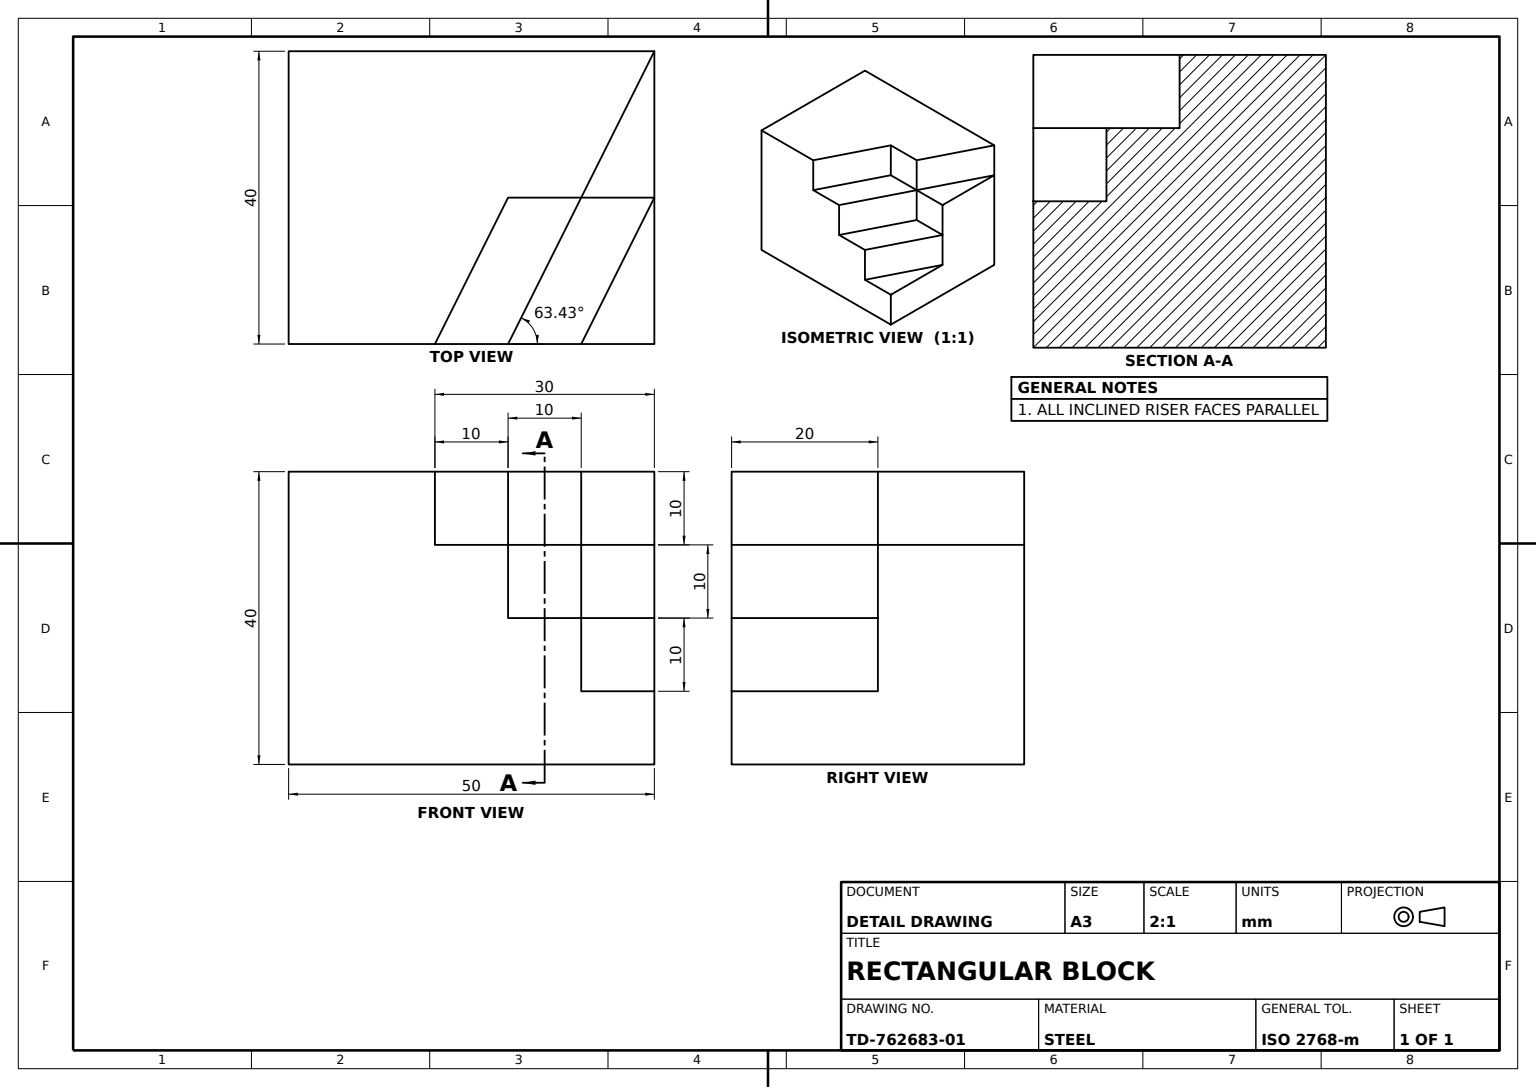
from build123d import *

# Parameters (mm, degrees)
BASE_BLOCK_PROFILE_W      = 50
BASE_BLOCK_PROFILE_H      = 40
BASE_BLOCK_50X40X40_DEPTH = 20
STEP_CUT_1_DEPTH          = 10
STEP_CUT_2_DEPTH          = 10
STEP_CUT_3_DEPTH          = 10


with BuildPart() as part:
    # Base Block Profile → Base Block 50x40x40 (new, symmetric)
    with BuildSketch(Plane(origin=(0, 0, 0), x_dir=(1, 0, 0), z_dir=(0, 1, 0))):
        Rectangle(BASE_BLOCK_PROFILE_W, BASE_BLOCK_PROFILE_H)
    extrude(amount=BASE_BLOCK_50X40X40_DEPTH, both=True)

    # Step Cut 1 Profile → Step Cut 1 (cut)
    with BuildSketch(Plane(origin=(0, 20, 0), x_dir=(1, 0, 0), z_dir=(0, 1, 0))):
        Polygon((25, 20), (15, 0), (5, 0), (-5, -20), (25, -20), align=None)
    extrude(amount=-STEP_CUT_1_DEPTH, mode=Mode.SUBTRACT)

    # Step Cut 2 Profile → Step Cut 2 (cut)
    with BuildSketch(Plane(origin=(0, 10, 0), x_dir=(1, 0, 0), z_dir=(0, 1, 0))):
        Polygon((25, 0), (15, 0), (5, -20), (25, -20), align=None)
    extrude(amount=-STEP_CUT_2_DEPTH, mode=Mode.SUBTRACT)

    # Step Cut 3 Profile → Step Cut 3 (cut)
    with BuildSketch(Plane(origin=(0, 0, 0), x_dir=(1, 0, 0), z_dir=(0, 1, 0))):
        Polygon((25, -20), (25, 0), (15, -20), align=None)
    extrude(amount=-STEP_CUT_3_DEPTH, mode=Mode.SUBTRACT)


solid = part.part
